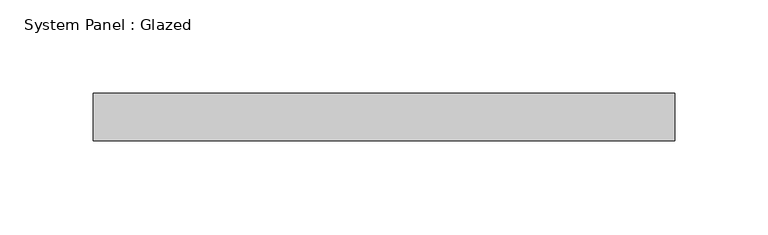
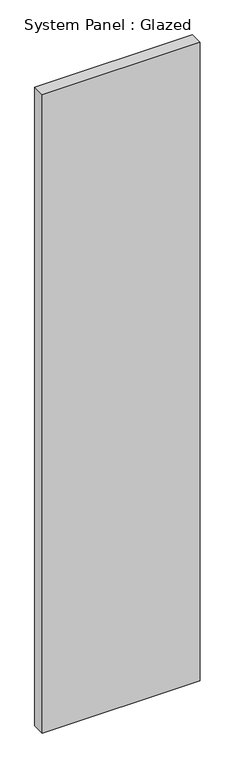
"""IFC4 building model written with IfcOpenShell, lengths in millimetres: plate geometry, System Panel : Glazed."""

from ifc_helpers import new_model, si_unit, origin, origin_with_axes, place, context, project, spatial, polyline, outline, extrude, source, transform, mapped, element, save


def system_panel_glazed_fe9977b0(model_context):
    return source(origin(), model_context, "Body", "SweptSolid", [
        extrude(outline(polyline([(155.575, 19.05), (-155.575, 19.05), (-155.575, 44.45), (155.575, 44.45), (155.575, 19.05)])), origin_with_axes(), (0.0, 0.0, 1.0), 1330.1797686),
    ])


if __name__ == "__main__":
    model = new_model("IFC4")
    model_context = context("Model", 3, world=origin())
    ifc_project = project(units=[si_unit("LENGTHUNIT", "METRE", prefix="MILLI")], contexts=[model_context])
    site = spatial("IfcSite", under=ifc_project)
    building = spatial("IfcBuilding", under=site)
    placement = place(None, origin())
    system_panel_glazed_shape = system_panel_glazed_fe9977b0(model_context)
    element("IfcPlate", 1, ObjectType="System Panel : Glazed", at=placement, inside=building, context=model_context, shape_type="MappedRepresentation", body=[
        mapped(system_panel_glazed_shape, transform((0.0, 0.0, 0.0), x_axis=(1.0, 0.0, 0.0), y_axis=(0.0, 1.0, 0.0), z_axis=(0.0, 0.0, 1.0))),
    ])
    save(model, "model.ifc")

# Revit data of these elements
# Type "System Panel : Glazed"
#   Construction Type Id = "GSP4R"
#   Analytic Construction = "1/8 in Pilkington single glazing"
#   Visual Light Transmittance = 0.9
#   Solar Heat Gain Coefficient = 0.86
#   Heat Transfer Coefficient (U) = 1.18115 BTU/(h·ft²·°F)
#   Define Thermal Properties by = 1
# Element 1 (IfcPlate, "System Panel : Glazed")
#   Materials on its faces: "Glass"
# Materials
#   "Glass": class "Glass", colour RGB 0 128 192, transparency 0.75, Description = "Soda Lime Glass", Cost = 0
